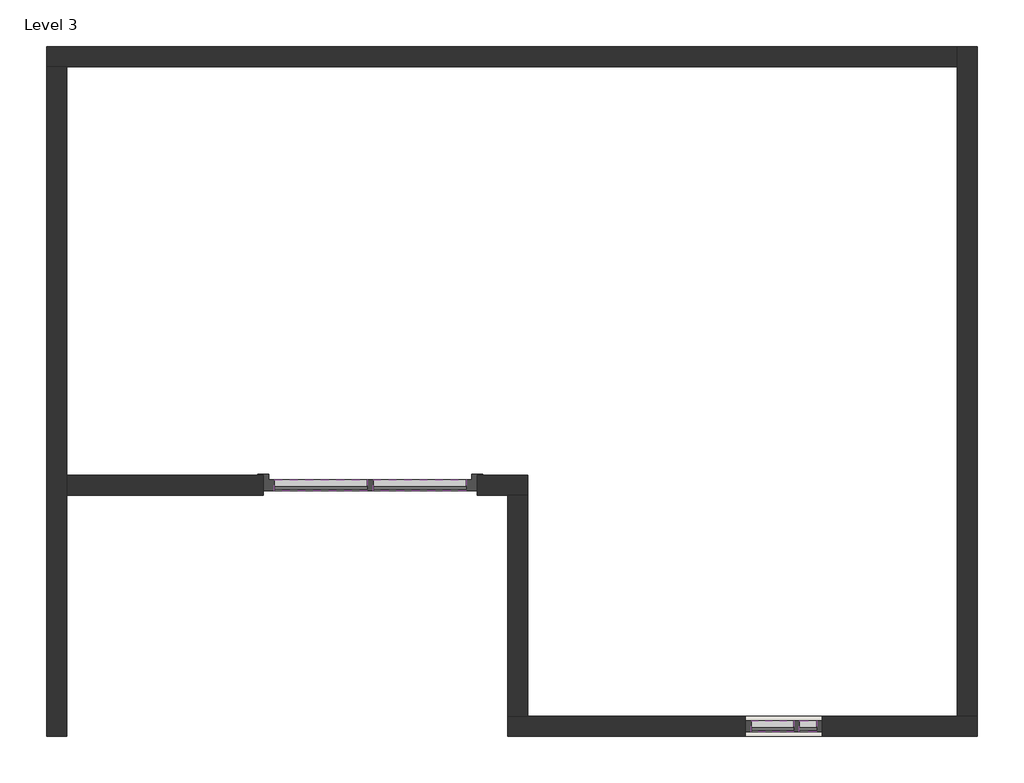
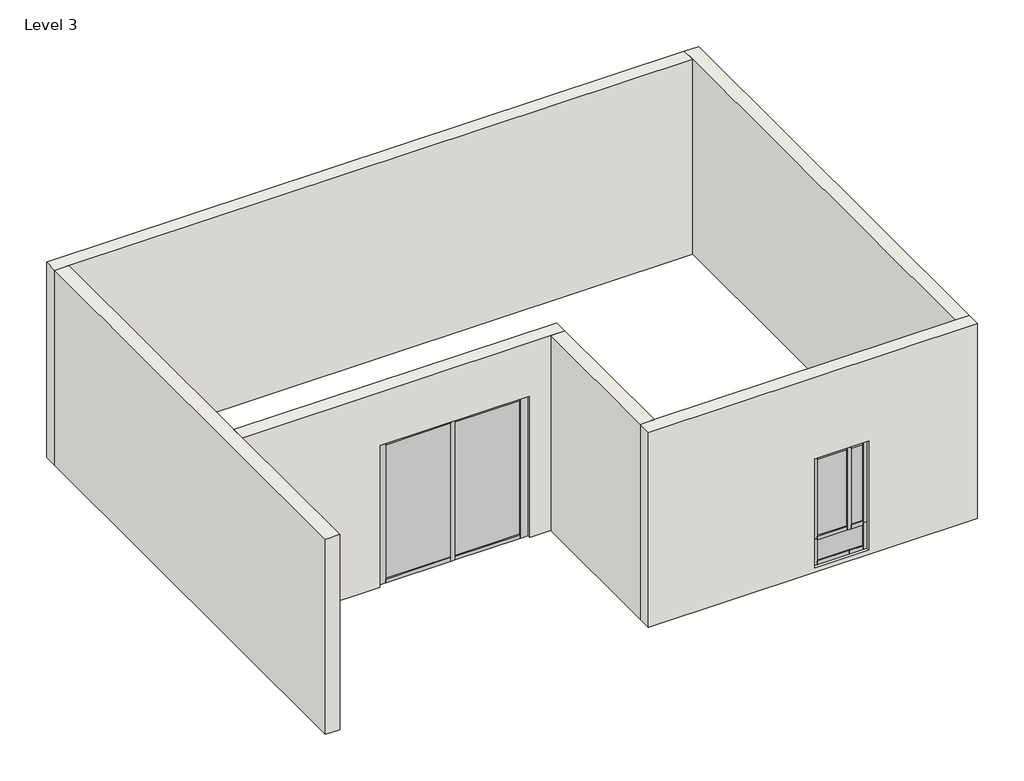
# One storey: 18 members, 6 walls, 5 plates.
"""IFC4 building model written with IfcOpenShell, lengths in millimetres."""

from ifc_helpers import new_model, si_unit, frame, origin, place, context, project, spatial, polyline, outline, extrude, faceted_brep, transform, mapped, element, save
from components import member_cc254986, member_d13a5c2f, member_f0fea5a5, member_4de4f528, member_15823cb3, member_bb91b9b7, member_6a4379ac, member_1d451195, member_d97a949f, member_fe2d9451, member_1750048d, member_f7b56663, system_panel_glazed_6ba90871, system_panel_glazed_a3b4e73b, system_panel_glazed_43c0a51f, system_panel_glazed_a3f5704d

model = new_model("IFC4")

# Units and contexts
model_context = context("Model", 3, world=origin())
ifc_project = project(units=[si_unit("LENGTHUNIT", "METRE", prefix="MILLI")], contexts=[model_context])

# Site, building, storey
site = spatial("IfcSite", under=ifc_project)
building = spatial("IfcBuilding", under=site)
storey = spatial("IfcBuildingStorey", under=building, Name="Level 3", Elevation=3200.4)

# Members
placement = place(None, origin())
member_shape = member_cc254986(model_context)
element("IfcMember", 1, ObjectType="L Corner Mullion : 5\" x 5\" Corner", at=placement, inside=storey, context=model_context, shape_type="MappedRepresentation", body=[
    mapped(member_shape, transform((-7394.7379854, -2948.9506821, 3200.4), x_axis=(-1.0, 0.0, 0.0), y_axis=(0.0, 1.0, 0.0), z_axis=(0.0, 0.0, -1.0))),
])
element("IfcMember", 2, ObjectType="L Corner Mullion : 5\" x 5\" Corner", at=placement, inside=storey, context=model_context, shape_type="MappedRepresentation", body=[
    mapped(member_shape, transform((-4956.3379854, -2948.9506821, 5638.8), x_axis=(1.0, 0.0, 0.0), y_axis=(0.0, 1.0, 0.0), z_axis=(0.0, 0.0, 1.0))),
])
member_2_shape = member_d13a5c2f(model_context)
element("IfcMember", 3, ObjectType="Rectangular Mullion : 2.5\" x 5\" rectangular", at=placement, inside=storey, context=model_context, shape_type="MappedRepresentation", body=[
    mapped(member_2_shape, transform((-7267.7379854, -2948.9506821, 5638.8), x_axis=(0.0, 0.0, 1.0), y_axis=(0.0, 1.0, 0.0), z_axis=(-1.0, 0.0, 0.0))),
])
element("IfcMember", 4, ObjectType="Rectangular Mullion : 2.5\" x 5\" rectangular", at=placement, inside=storey, context=model_context, shape_type="MappedRepresentation", body=[
    mapped(member_2_shape, transform((-6143.7879854, -2948.9506821, 5638.8), x_axis=(0.0, 0.0, 1.0), y_axis=(0.0, 1.0, 0.0), z_axis=(-1.0, 0.0, 0.0))),
])
element("IfcMember", 5, ObjectType="Rectangular Mullion : 2.5\" x 5\" rectangular", at=placement, inside=storey, context=model_context, shape_type="MappedRepresentation", body=[
    mapped(member_2_shape, transform((-5083.3379854, -2948.9506821, 3200.4), x_axis=(0.0, 0.0, -1.0), y_axis=(0.0, 1.0, 0.0), z_axis=(1.0, 0.0, 0.0))),
])
element("IfcMember", 6, ObjectType="Rectangular Mullion : 2.5\" x 5\" rectangular", at=placement, inside=storey, context=model_context, shape_type="MappedRepresentation", body=[
    mapped(member_2_shape, transform((-6207.2879854, -2948.9506821, 3200.4), x_axis=(0.0, 0.0, -1.0), y_axis=(0.0, 1.0, 0.0), z_axis=(1.0, 0.0, 0.0))),
])
member_3_shape = member_f0fea5a5(model_context)
element("IfcMember", 7, ObjectType="Rectangular Mullion : 2.5\" x 5\" rectangular", at=placement, inside=storey, context=model_context, shape_type="MappedRepresentation", body=[
    mapped(member_3_shape, transform((-6175.5379854, -2948.9506821, 3200.4), x_axis=(-1.0, 0.0, 0.0), y_axis=(0.0, 1.0, 0.0), z_axis=(0.0, 0.0, -1.0))),
])
member_4_shape = member_4de4f528(model_context)
element("IfcMember", 8, ObjectType="Rectangular Mullion : 2.5\" x 5\" rectangular", at=placement, inside=storey, context=model_context, shape_type="MappedRepresentation", body=[
    mapped(member_4_shape, transform((-1032.0379854, -5692.1506821, 5149.0315053), x_axis=(1.0, 0.0, 0.0), y_axis=(0.0, 1.0, 0.0), z_axis=(0.0, 0.0, 1.0))),
])
member_5_shape = member_15823cb3(model_context)
element("IfcMember", 9, ObjectType="Rectangular Mullion : 2.5\" x 5\" rectangular", at=placement, inside=storey, context=model_context, shape_type="MappedRepresentation", body=[
    mapped(member_5_shape, transform((-1906.102741, -5692.1506821, 3276.6), x_axis=(-1.0, 0.0, 0.0), y_axis=(0.0, 1.0, 0.0), z_axis=(0.0, 0.0, -1.0))),
])
element("IfcMember", 10, ObjectType="Rectangular Mullion : 2.5\" x 5\" rectangular", at=placement, inside=storey, context=model_context, shape_type="MappedRepresentation", body=[
    mapped(member_4_shape, transform((-1906.102741, -5692.1506821, 3733.8), x_axis=(-1.0, 0.0, 0.0), y_axis=(0.0, 1.0, 0.0), z_axis=(0.0, 0.0, -1.0))),
])
element("IfcMember", 11, ObjectType="Rectangular Mullion : 2.5\" x 5\" rectangular", at=placement, inside=storey, context=model_context, shape_type="MappedRepresentation", body=[
    mapped(member_5_shape, transform((-1032.0379854, -5692.1506821, 3733.8), x_axis=(1.0, 0.0, 0.0), y_axis=(0.0, 1.0, 0.0), z_axis=(0.0, 0.0, 1.0))),
])
member_6_shape = member_bb91b9b7(model_context)
element("IfcMember", 12, ObjectType="Rectangular Mullion : 2.5\" x 5\" rectangular", at=placement, inside=storey, context=model_context, shape_type="MappedRepresentation", body=[
    mapped(member_6_shape, transform((-1095.5379854, -5692.1506821, 3276.6), x_axis=(0.0, 0.0, -1.0), y_axis=(0.0, 1.0, 0.0), z_axis=(1.0, 0.0, 0.0))),
])
member_7_shape = member_6a4379ac(model_context)
element("IfcMember", 13, ObjectType="Rectangular Mullion : 2.5\" x 5\" rectangular", at=placement, inside=storey, context=model_context, shape_type="MappedRepresentation", body=[
    mapped(member_7_shape, transform((-1323.3929039, -5692.1506821, 3276.6), x_axis=(0.0, 0.0, -1.0), y_axis=(0.0, 1.0, 0.0), z_axis=(1.0, 0.0, 0.0))),
])
member_8_shape = member_1d451195(model_context)
element("IfcMember", 14, ObjectType="Rectangular Mullion : 2.5\" x 5\" rectangular", at=placement, inside=storey, context=model_context, shape_type="MappedRepresentation", body=[
    mapped(member_8_shape, transform((-1842.602741, -5692.1506821, 5149.0315053), x_axis=(0.0, 0.0, 1.0), y_axis=(0.0, 1.0, 0.0), z_axis=(-1.0, 0.0, 0.0))),
])
member_9_shape = member_d97a949f(model_context)
element("IfcMember", 15, ObjectType="Rectangular Mullion : 2.5\" x 5\" rectangular", at=placement, inside=storey, context=model_context, shape_type="MappedRepresentation", body=[
    mapped(member_9_shape, transform((-1291.6429039, -5692.1506821, 3733.8), x_axis=(0.0, 0.0, 1.0), y_axis=(0.0, 1.0, 0.0), z_axis=(-1.0, 0.0, 0.0))),
])
member_10_shape = member_fe2d9451(model_context)
element("IfcMember", 16, ObjectType="Rectangular Mullion : 2.5\" x 5\" rectangular", at=placement, inside=storey, context=model_context, shape_type="MappedRepresentation", body=[
    mapped(member_10_shape, transform((-1291.6429039, -5692.1506821, 5149.0315053), x_axis=(0.0, 0.0, 1.0), y_axis=(0.0, 1.0, 0.0), z_axis=(-1.0, 0.0, 0.0))),
])
member_11_shape = member_1750048d(model_context)
element("IfcMember", 17, ObjectType="Rectangular Mullion : 2.5\" x 5\" rectangular", at=placement, inside=storey, context=model_context, shape_type="MappedRepresentation", body=[
    mapped(member_11_shape, transform((-1842.602741, -5692.1506821, 3733.8), x_axis=(0.0, 0.0, 1.0), y_axis=(0.0, 1.0, 0.0), z_axis=(-1.0, 0.0, 0.0))),
])
member_12_shape = member_f7b56663(model_context)
element("IfcMember", 18, ObjectType="Rectangular Mullion : 2.5\" x 5\" rectangular", at=placement, inside=storey, context=model_context, shape_type="MappedRepresentation", body=[
    mapped(member_12_shape, transform((-1323.3929039, -5692.1506821, 3702.05), x_axis=(-1.0, 0.0, 0.0), y_axis=(0.0, 1.0, 0.0), z_axis=(0.0, 0.0, -1.0))),
])

# Plates
system_panel_glazed_shape = system_panel_glazed_6ba90871(model_context)
element("IfcPlate", 19, ObjectType="System Panel : Glazed", at=placement, inside=storey, context=model_context, shape_type="MappedRepresentation", body=[
    mapped(system_panel_glazed_shape, transform((-5613.5629854, -2948.9506821, 3263.9), x_axis=(-1.0, 0.0, 0.0), y_axis=(0.0, -1.0, 0.0), z_axis=(0.0, 0.0, 1.0))),
])
element("IfcPlate", 20, ObjectType="System Panel : Glazed", at=placement, inside=storey, context=model_context, shape_type="MappedRepresentation", body=[
    mapped(system_panel_glazed_shape, transform((-6737.5129854, -2948.9506821, 3263.9), x_axis=(-1.0, 0.0, 0.0), y_axis=(0.0, -1.0, 0.0), z_axis=(0.0, 0.0, 1.0))),
])
system_panel_glazed_2_shape = system_panel_glazed_a3b4e73b(model_context)
element("IfcPlate", 21, ObjectType="System Panel : Glazed", at=placement, inside=storey, context=model_context, shape_type="MappedRepresentation", body=[
    mapped(system_panel_glazed_2_shape, transform((-1469.0703632, -5692.1506821, 3340.1), x_axis=(-1.0, 0.0, 0.0), y_axis=(0.0, -1.0, 0.0), z_axis=(0.0, 0.0, 1.0))),
])
system_panel_glazed_3_shape = system_panel_glazed_43c0a51f(model_context)
element("IfcPlate", 22, ObjectType="System Panel : Glazed", at=placement, inside=storey, context=model_context, shape_type="MappedRepresentation", body=[
    mapped(system_panel_glazed_3_shape, transform((-1193.5904446, -5692.1506821, 3765.55), x_axis=(-1.0, 0.0, 0.0), y_axis=(0.0, -1.0, 0.0), z_axis=(0.0, 0.0, 1.0))),
])
system_panel_glazed_4_shape = system_panel_glazed_a3f5704d(model_context)
element("IfcPlate", 23, ObjectType="System Panel : Glazed", at=placement, inside=storey, context=model_context, shape_type="MappedRepresentation", body=[
    mapped(system_panel_glazed_4_shape, transform((-1598.8728225, -5692.1506821, 3765.55), x_axis=(-1.0, 0.0, 0.0), y_axis=(0.0, -1.0, 0.0), z_axis=(0.0, 0.0, 1.0))),
])

# Walls
element("IfcWall", 24, ObjectType="9\" wall", at=placement, inside=storey, context=model_context, shape_type="Brep", body=[
    faceted_brep([(-9858.5379854, 1813.5493179, 3200.4), (-9629.9379854, 1813.5493179, 3200.4), (504.6620146, 1813.5493179, 3200.4), (504.6620146, 1813.5493179, 6553.2), (-9629.9379854, 1813.5493179, 6553.2), (-9858.5379854, 1813.5493179, 6553.2), (-9858.5379854, 2042.1493179, 3200.4), (-9858.5379854, 2042.1493179, 6553.2), (504.6620146, 2042.1493179, 6553.2), (504.6620146, 2042.1493179, 3200.4)], [[[0, 1, 2, 3, 4, 5]], [[6, 7, 8, 9]], [[2, 1, 0, 6, 9]], [[5, 4, 3, 8, 7]], [[0, 5, 7, 6]], [[3, 2, 9, 8]]]),
])
element("IfcWall", 25, ObjectType="9\" wall", at=placement, inside=storey, context=model_context, shape_type="Brep", body=[
    faceted_brep([(-9629.9379854, -5806.4506821, 3200.4), (-9629.9379854, -3063.2506821, 3200.4), (-9629.9379854, -2834.6506821, 3200.4), (-9629.9379854, 1813.5493179, 3200.4), (-9629.9379854, 1813.5493179, 6553.2), (-9629.9379854, -2834.6506821, 6553.2), (-9629.9379854, -3063.2506821, 6553.2), (-9629.9379854, -5806.4506821, 6553.2), (-9858.5379854, -5806.4506821, 3200.4), (-9858.5379854, -5806.4506821, 6553.2), (-9858.5379854, 1813.5493179, 6553.2), (-9858.5379854, 1813.5493179, 3200.4)], [[[0, 1, 2, 3, 4, 5, 6, 7]], [[8, 9, 10, 11]], [[3, 2, 1, 0, 8, 11]], [[7, 6, 5, 4, 10, 9]], [[0, 7, 9, 8]], [[4, 3, 11, 10]]]),
])
element("IfcWall", 26, ObjectType="9\" wall", at=placement, inside=storey, context=model_context, shape_type="Brep", body=[
    faceted_brep([(733.2620146, -5577.8506821, 3200.4), (504.6620146, -5577.8506821, 3200.4), (-4384.8379854, -5577.8506821, 3200.4), (-4613.4379854, -5577.8506821, 3200.4), (-4613.4379854, -5577.8506821, 6553.2), (-4384.8379854, -5577.8506821, 6553.2), (504.6620146, -5577.8506821, 6553.2), (733.2620146, -5577.8506821, 6553.2), (-1032.0379854, -5577.8506821, 3276.6), (-1032.0379854, -5577.8506821, 5149.0315053), (-1906.102741, -5577.8506821, 5149.0315053), (-1906.102741, -5577.8506821, 3276.6), (-4613.4379854, -5806.4506821, 3200.4), (733.2620146, -5806.4506821, 3200.4), (733.2620146, -5806.4506821, 6553.2), (-4613.4379854, -5806.4506821, 6553.2), (-1032.0379854, -5806.4506821, 5149.0315053), (-1032.0379854, -5806.4506821, 3276.6), (-1906.102741, -5806.4506821, 3276.6), (-1906.102741, -5806.4506821, 5149.0315053)], [[[0, 1, 2, 3, 4, 5, 6, 7], [8, 9, 10, 11]], [[12, 13, 14, 15], [16, 17, 18, 19]], [[3, 2, 1, 0, 13, 12]], [[7, 6, 5, 4, 15, 14]], [[0, 7, 14, 13]], [[4, 3, 12, 15]], [[8, 17, 16, 9]], [[9, 16, 19, 10]], [[10, 19, 18, 11]], [[17, 8, 11, 18]]]),
])
element("IfcWall", 27, ObjectType="9\" wall", at=placement, inside=storey, context=model_context, shape_type="Brep", body=[
    faceted_brep([(504.6620146, 2042.1493179, 3200.4), (504.6620146, 1813.5493179, 3200.4), (504.6620146, -5577.8506821, 3200.4), (504.6620146, -5577.8506821, 6553.2), (504.6620146, 1813.5493179, 6553.2), (504.6620146, 2042.1493179, 6553.2), (733.2620146, 2042.1493179, 3200.4), (733.2620146, 2042.1493179, 6553.2), (733.2620146, -5577.8506821, 6553.2), (733.2620146, -5577.8506821, 3200.4)], [[[0, 1, 2, 3, 4, 5]], [[6, 7, 8, 9]], [[2, 1, 0, 6, 9]], [[5, 4, 3, 8, 7]], [[0, 5, 7, 6]], [[3, 2, 9, 8]]]),
])
element("IfcWall", 28, ObjectType="9\" wall", at=placement, inside=storey, context=model_context, shape_type="Brep", body=[
    faceted_brep([(-4384.8379854, -3063.2506821, 6553.2), (-4613.4379854, -3063.2506821, 6553.2), (-9629.9379854, -3063.2506821, 6553.2), (-9629.9379854, -3063.2506821, 3200.4), (-7394.7379854, -3063.2506821, 3200.4), (-7394.7379854, -3063.2506821, 5638.8), (-4956.3379854, -3063.2506821, 5638.8), (-4956.3379854, -3063.2506821, 3200.4), (-4613.4379854, -3063.2506821, 3200.4), (-4384.8379854, -3063.2506821, 3200.4), (-9629.9379854, -2834.6506821, 6553.2), (-4384.8379854, -2834.6506821, 6553.2), (-4384.8379854, -2834.6506821, 3200.4), (-4956.3379854, -2834.6506821, 3200.4), (-4956.3379854, -2834.6506821, 5638.8), (-7394.7379854, -2834.6506821, 5638.8), (-7394.7379854, -2834.6506821, 3200.4), (-9629.9379854, -2834.6506821, 3200.4)], [[[0, 1, 2, 3, 4, 5, 6, 7, 8, 9]], [[10, 11, 12, 13, 14, 15, 16, 17]], [[12, 9, 8, 7, 13]], [[3, 17, 16, 4]], [[2, 1, 0, 11, 10]], [[0, 9, 12, 11]], [[3, 2, 10, 17]], [[6, 14, 13, 7]], [[14, 6, 5, 15]], [[15, 5, 4, 16]]]),
])
element("IfcWall", 29, ObjectType="9\" wall", at=placement, inside=storey, context=model_context, shape_type="SweptSolid", body=[
    extrude(outline(polyline([(-4613.4379854, -5577.8506821), (-4613.4379854, -3063.2506821), (-4384.8379854, -3063.2506821), (-4384.8379854, -5577.8506821), (-4613.4379854, -5577.8506821)])), frame((0.0, 0.0, 3200.4), z_axis=(0.0, 0.0, 1.0), x_axis=(1.0, 0.0, 0.0)), (0.0, 0.0, 1.0), 3352.8),
])

save(model, "model.ifc")

# Revit data of these elements
# Type "L Corner Mullion : 5\" x 5\" Corner"
#   built-in parameter 1007355 = 0.416667 (stored number, unit not read)
#   built-in parameter 1007354 = 0.416667 (stored number, unit not read)
#   built-in parameter 1007304 = 0.416667 (stored number, unit not read)
# Type "Rectangular Mullion : 2.5\" x 5\" rectangular"
#   built-in parameter 1007304 = 0.416667 (stored number, unit not read)
#   built-in parameter 1007301 = 0.104167 (stored number, unit not read)
#   built-in parameter 1007300 = 0.104167 (stored number, unit not read)
# Type "System Panel : Glazed"
#   Construction Type Id = "GSP4R"
#   Analytic Construction = "1/8 in Pilkington single glazing"
#   Visual Light Transmittance = 0.9
#   Solar Heat Gain Coefficient = 0.86
#   Heat Transfer Coefficient (U) = 1.18115 BTU/(h·ft²·°F)
#   Define Thermal Properties by = 1
# Type "9\" wall"
#   Assembly Code = "B2010"
# Elements 1, 2 (IfcMember, "L Corner Mullion : 5\" x 5\" Corner")
#   Phase Created = New Construction
#   Materials on its faces: "mullions"
# Elements 3, 4, 5, 6, 7, 8, 9, 10, 11, 12, 13, 14, 15, 16, 17, 18 (IfcMember, "Rectangular Mullion : 2.5\" x 5\" rectangular")
#   Phase Created = New Construction
#   Materials on its faces: "mullions"
# Elements 19, 20, 21, 22, 23 (IfcPlate, "System Panel : Glazed")
#   Phase Created = New Construction
#   Materials on its faces: "Glass"
# Elements 24, 25, 26, 27, 28, 29 (IfcWall, "9\" wall")
#   Top Offset = 1' - 0"
#   Base Offset = 0' - 0"
#   wall height = 11' - 0"
#   Phase Created = New Construction
#   Base Constraint = Level 3
#   Top Constraint = Level 4
# Materials
#   "mullions": class "Generic", colour RGB 120 120 120, transparency 0, Cost = 0
#   "Glass": class "Glass", colour RGB 0 128 192, transparency 0.75, Description = "Soda Lime Glass", Cost = 0
